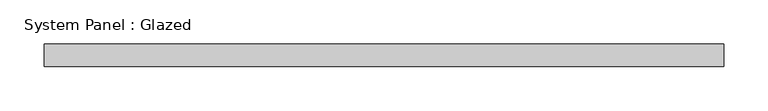
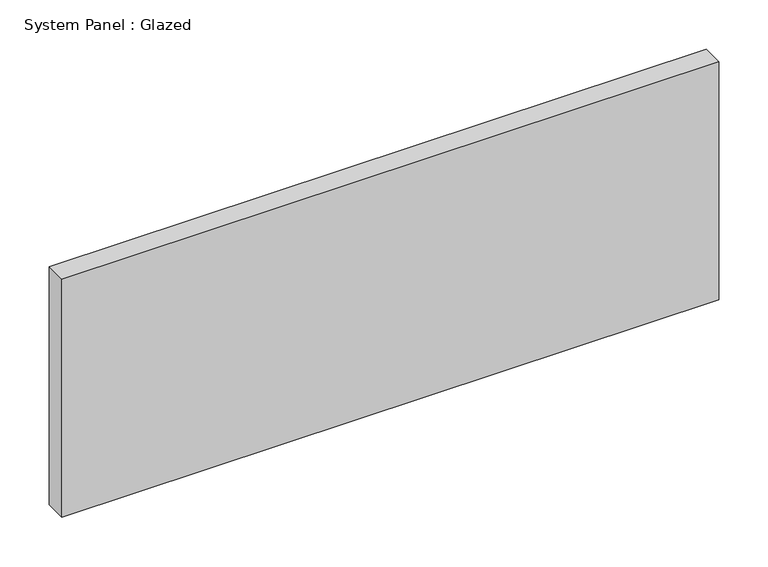
"""IFC4 building model written with IfcOpenShell, lengths in millimetres: plate geometry, System Panel : Glazed."""

from ifc_helpers import new_model, si_unit, origin, origin_with_axes, place, context, project, spatial, polyline, outline, extrude, source, transform, mapped, element, save


def system_panel_glazed_aaa2c267(model_context):
    return source(origin(), model_context, "Body", "SweptSolid", [
        extrude(outline(polyline([(383.50825, 19.05), (-383.50825, 19.05), (-383.50825, 44.45), (383.50825, 44.45), (383.50825, 19.05)])), origin_with_axes(), (0.0, 0.0, 1.0), 293.9415),
    ])


if __name__ == "__main__":
    model = new_model("IFC4")
    model_context = context("Model", 3, world=origin())
    ifc_project = project(units=[si_unit("LENGTHUNIT", "METRE", prefix="MILLI")], contexts=[model_context])
    site = spatial("IfcSite", under=ifc_project)
    building = spatial("IfcBuilding", under=site)
    placement = place(None, origin())
    system_panel_glazed_shape = system_panel_glazed_aaa2c267(model_context)
    element("IfcPlate", 1, ObjectType="System Panel : Glazed", at=placement, inside=building, context=model_context, shape_type="MappedRepresentation", body=[
        mapped(system_panel_glazed_shape, transform((0.0, 0.0, 0.0), x_axis=(1.0, 0.0, 0.0), y_axis=(0.0, 1.0, 0.0), z_axis=(0.0, 0.0, 1.0))),
    ])
    save(model, "model.ifc")

# Revit data of these elements
# Type "System Panel : Glazed"
#   Construction Type Id = "GSP4R"
#   Analytic Construction = "1/8 in Pilkington single glazing"
#   Visual Light Transmittance = 0.9
#   Solar Heat Gain Coefficient = 0.86
#   Heat Transfer Coefficient (U) = 1.18115 BTU/(h·ft²·°F)
#   Define Thermal Properties by = 1
# Element 1 (IfcPlate, "System Panel : Glazed")
#   Materials on its faces: "Glass"
# Materials
#   "Glass": class "Glass", colour RGB 0 128 192, transparency 0.75, Description = "Soda Lime Glass", Cost = 0
